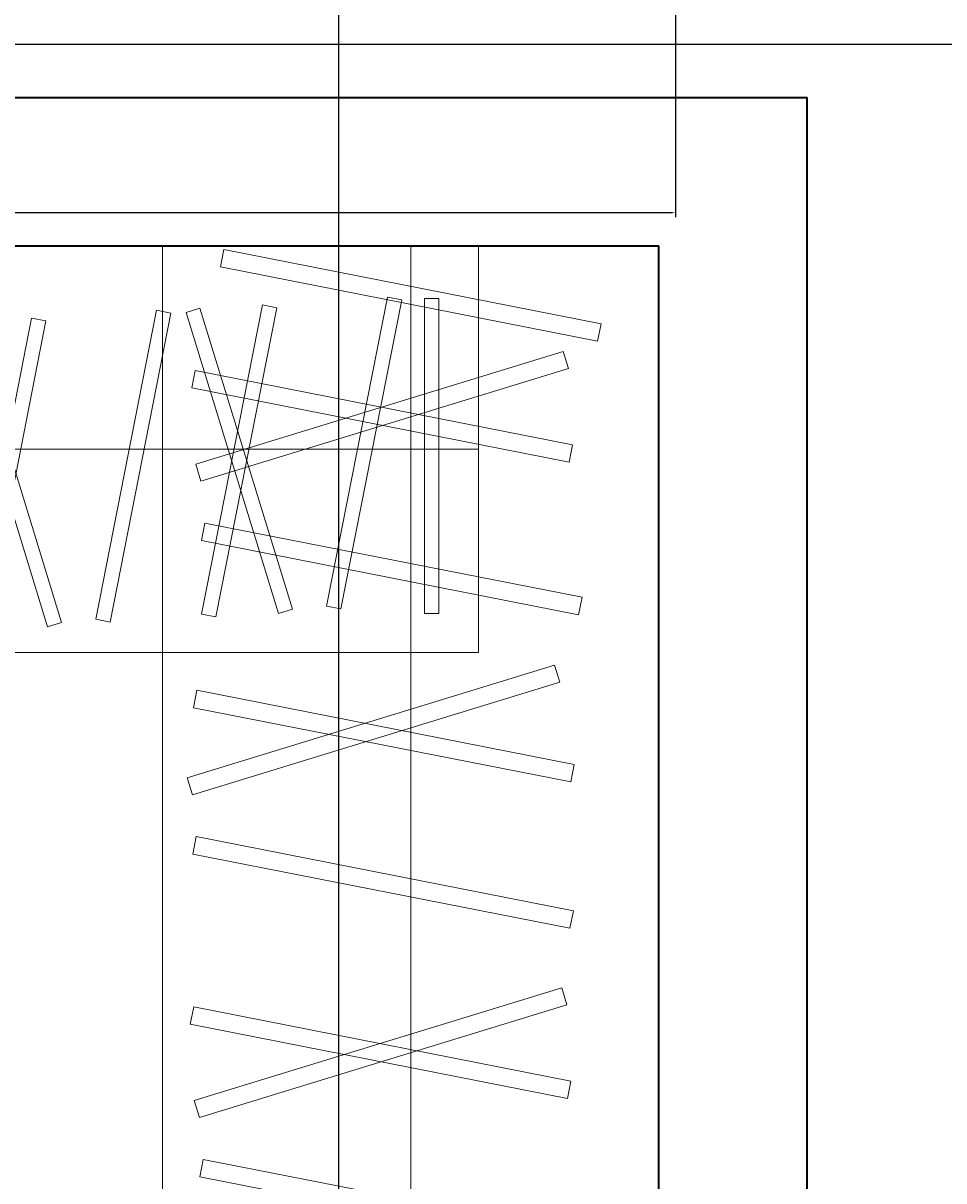
# Model space of a CAD drawing. Units: inches. Extents: x -61 to 1599, y -1316 to 257.
# Tile 66 of 204: x 203 to 240, y -213 to -166. Entities that reach past the tile are written whole.
import ezdxf

# ---------------------------------------------------------------- set-up
doc = ezdxf.new("R2010")
doc.units = ezdxf.units.IN
doc.header["$MEASUREMENT"] = 0
for name, color, linetype, lineweight in [('A-ANNO-DIMS', 2, 'Continuous', 18), ('A-FLOR-CASE', 8, 'Continuous', 18), ('WALLS', 4, 'Continuous', 35)]:
    doc.layers.add(name, color=color, linetype=linetype, lineweight=lineweight)
doc.styles.get("Standard").update_dxf_attribs({"font": 'arial.ttf'})
doc.dimstyles.get("Standard").update_dxf_attribs({"dimtxt": 0.18, "dimasz": 0.18, "dimexe": 0.18, "dimexo": 0.0625, "dimgap": 0.09, "dimtad": 0, "dimtih": 1, "dimtoh": 1, "dimdec": 0, "dimzin": 0, "dimdsep": 46, "dimlunit": 3, "dimtxsty": 'Standard', "dimcen": 0.09, "dimadec": 0, "dimazin": 0, "dimtfac": 1, "dimtdec": 0, "dimtofl": 0, "dimtmove": 0, "dimatfit": 3, "dimfxl": 1, "dimtolj": 1, "dimtzin": 0, "dimarcsym": 0})

# ---------------------------------------------------------------- blocks, each defined once
blk = doc.blocks.new('WARDROBE-HANGING')
blk.add_line((10.047, 0), (10.047, 68))
for points in [[(20.094, 0), (0, 0), (0, 68), (20.094, 68)], [(2.482, 67.852), (17.751, 64.849), (17.612, 64.142), (2.343, 67.146)], [(1.346, 59.162), (16.221, 63.731), (16.432, 63.043), (1.557, 58.474)], [(1.325, 62.957), (16.593, 59.954), (16.454, 59.247), (1.186, 62.251)], [(1.713, 56.784), (16.981, 53.781), (16.842, 53.074), (1.574, 56.078)], [(0.997, 46.467), (15.872, 51.036), (16.084, 50.348), (1.209, 45.779)], [(1.394, 50.014), (16.662, 47.011), (16.523, 46.305), (1.255, 49.308)], [(1.365, 44.09), (16.633, 41.086), (16.494, 40.38), (1.226, 43.383)], [(1.283, 33.408), (16.158, 37.977), (16.37, 37.289), (1.495, 32.72)], [(1.262, 37.203), (16.53, 34.2), (16.391, 33.493), (1.123, 36.497)], [(1.651, 31.03), (16.919, 28.027), (16.78, 27.32), (1.512, 30.324)]]:
    blk.add_lwpolyline(points, close=True)
blk = doc.blocks.new('WARDROBE-HANGING-2')
blk.add_line((55.703, 8.23), (0, 8.23))
for points in [[(55.703, 16.46), (55.703, 0), (0, 0), (0, 16.46)], [(0.121, 2.033), (2.581, 14.541), (3.16, 14.427), (0.7, 1.92)], [(44.491, 1.561), (46.952, 14.069), (47.53, 13.955), (45.07, 1.448)], [(49.548, 1.88), (52.008, 14.387), (52.587, 14.273), (50.127, 1.766)], [(54.096, 14.328), (54.096, 1.581), (53.506, 1.581), (53.506, 14.328)], [(4.131, 1.085), (6.591, 13.592), (7.17, 13.478), (4.709, 0.971)], [(9.187, 1.403), (11.648, 13.911), (12.226, 13.797), (9.766, 1.289)], [(14.733, 1.142), (17.193, 13.649), (17.772, 13.535), (15.312, 1.028)], [(19.586, 1.118), (22.047, 13.625), (22.625, 13.511), (20.165, 1.004)], [(30.284, 1.352), (32.745, 13.859), (33.323, 13.745), (30.863, 1.238)], [(40.204, 1.348), (42.664, 13.855), (43.243, 13.742), (40.782, 1.234)], [(47.6, 1.579), (43.858, 13.764), (44.421, 13.937), (48.164, 1.752)], [(7.24, 1.102), (3.497, 13.288), (4.061, 13.461), (7.804, 1.276)], [(17.639, 0.817), (13.896, 13.002), (14.46, 13.175), (18.203, 0.99)], [(28.337, 1.051), (24.594, 13.236), (25.158, 13.409), (28.901, 1.224)], [(25.228, 1.034), (27.688, 13.541), (28.267, 13.427), (25.806, 0.92)], [(38.256, 1.047), (34.513, 13.232), (35.077, 13.406), (38.82, 1.221)], [(35.147, 1.03), (37.607, 13.537), (38.186, 13.423), (35.726, 0.916)]]:
    blk.add_lwpolyline(points, close=True)
blk = doc.blocks.new('*D670')
at = {"layer": 'A-ANNO-DIMS', "color": 0, "lineweight": -2, "transparency": 16777216}
for p, q in [((145.375, -161.442), (145.375, -174.159)), ((229.375, -161.442), (229.375, -174.159)), ((145.555, -173.979), (186.47, -173.979)), ((229.195, -173.979), (188.279, -173.979))]:
    blk.add_line(p, q, dxfattribs=at)
at = {"layer": 'A-ANNO-DIMS', "color": 0, "transparency": 16777216}
for points in [[(145.555, -173.949), (145.555, -174.009), (145.375, -173.979)], [(229.195, -173.949), (229.195, -174.009), (229.375, -173.979)]]:
    blk.add_solid(points, dxfattribs=at)
at = {"layer": 'DEFPOINTS', "color": 0, "transparency": 16777216}
for p in [(145.375, -161.379), (229.375, -161.379), (229.375, -173.979)]:
    blk.add_point(p, dxfattribs=at)
at = {"layer": 'A-ANNO-DIMS', "color": 0, "transparency": 16777216, "insert": (187.375, -173.979), "char_height": 0.18, "attachment_point": 5}
blk.add_mtext('\\A1;SOFA 84 TYP.', dxfattribs=at)
blk = doc.blocks.new('*D687')
at = {"layer": 'A-ANNO-DIMS', "color": 0, "lineweight": -2, "transparency": 16777216}
for p, q in [((289.418, 181.677), (-61.077, 181.677)), ((-60.897, 181.497), (-60.897, -528.952)), ((-60.897, -1239.765), (-60.897, -529.316)), ((319.64, -1239.945), (-61.077, -1239.945))]:
    blk.add_line(p, q, dxfattribs=at)
at = {"layer": 'A-ANNO-DIMS', "color": 0, "transparency": 16777216}
for points in [[(-60.927, 181.497), (-60.867, 181.497), (-60.897, 181.677)], [(-60.927, -1239.765), (-60.867, -1239.765), (-60.897, -1239.945)]]:
    blk.add_solid(points, dxfattribs=at)
at = {"layer": 'DEFPOINTS', "color": 0, "transparency": 16777216}
for p in [(289.481, 181.677), (-60.897, -1239.945), (319.703, -1239.945)]:
    blk.add_point(p, dxfattribs=at)
at = {"layer": 'A-ANNO-DIMS', "color": 0, "transparency": 16777216, "insert": (-60.897, -529.134), "char_height": 0.18, "attachment_point": 5}
blk.add_mtext('\\A1;1421.6', dxfattribs=at)
blk = doc.blocks.new('*D699')
at = {"layer": 'A-ANNO-DIMS', "color": 0, "lineweight": -2, "transparency": 16777216}
for p, q in [((835.64, -167.169), (-61.077, -167.169)), ((-60.897, -167.349), (-60.897, -306.726)), ((-60.897, -446.466), (-60.897, -307.09)), ((841.64, -446.646), (-61.077, -446.646))]:
    blk.add_line(p, q, dxfattribs=at)
at = {"layer": 'A-ANNO-DIMS', "color": 0, "transparency": 16777216}
for points in [[(-60.927, -167.349), (-60.867, -167.349), (-60.897, -167.169)], [(-60.927, -446.466), (-60.867, -446.466), (-60.897, -446.646)]]:
    blk.add_solid(points, dxfattribs=at)
at = {"layer": 'DEFPOINTS', "color": 0, "transparency": 16777216}
for p in [(835.703, -167.169), (-60.897, -446.646), (841.703, -446.646)]:
    blk.add_point(p, dxfattribs=at)
at = {"layer": 'A-ANNO-DIMS', "color": 0, "transparency": 16777216, "insert": (-60.897, -306.908), "char_height": 0.18, "attachment_point": 5}
blk.add_mtext('\\A1;279.5', dxfattribs=at)
blk = doc.blocks.new('*D701')
at = {"layer": 'A-ANNO-DIMS', "color": 0, "lineweight": -2, "transparency": 16777216}
for p, q in [((215.752, -616.882), (215.752, 257.457)), ((215.932, 257.277), (233.924, 257.277)), ((252.702, 257.277), (234.711, 257.277)), ((252.882, -616.882), (252.882, 257.457))]:
    blk.add_line(p, q, dxfattribs=at)
at = {"layer": 'A-ANNO-DIMS', "color": 0, "transparency": 16777216}
for points in [[(215.932, 257.307), (215.932, 257.247), (215.752, 257.277)], [(252.702, 257.307), (252.702, 257.247), (252.882, 257.277)]]:
    blk.add_solid(points, dxfattribs=at)
at = {"layer": 'DEFPOINTS', "color": 0, "transparency": 16777216}
for p in [(252.882, 257.277), (215.752, -616.945), (252.882, -616.945)]:
    blk.add_point(p, dxfattribs=at)
at = {"layer": 'A-ANNO-DIMS', "color": 0, "transparency": 16777216, "insert": (234.317, 257.277), "char_height": 0.18, "attachment_point": 5}
blk.add_mtext('\\A1;37.13', dxfattribs=at)

msp = doc.modelspace()

# ---------------------------------------------------------------- linework, layer by layer
at = {"layer": 'WALLS'}
for p, q in [((119.7028, -169.3229), (234.7028, -169.3229)), ((234.7028, -282.3229), (234.7028, -169.3229)), ((165.7028, -175.3229), (228.7028, -175.3229)), ((228.7028, -282.3229), (228.7028, -175.3229))]:
    msp.add_line(p, q, dxfattribs=at)

# ---------------------------------------------------------------- block references
at = {"layer": 'A-FLOR-CASE'}
for name, p in [('WARDROBE-HANGING-2', (165.703, -191.783)), ('WARDROBE-HANGING', (208.609, -243.323))]:
    msp.add_blockref(name, p, dxfattribs=at)

# ---------------------------------------------------------------- dimensions: what is measured, and where the dimension line sits
at = {"layer": 'A-ANNO-DIMS'}
dim = msp.add_linear_dim(base=(252.8825, 257.2771), p1=(215.7521, -616.9446), p2=(252.8825, -616.9446), dimstyle='Standard', override={"dimdec": 2, "dimlfac": 1, "dimrnd": 0, "dimzin": 0, "dimdsep": 46, "dimlunit": 2}, dxfattribs=at)
dim.commit()
dim.dimension.update_dxf_attribs({"geometry": '*D701', "text_midpoint": (234.3173, 257.2771)})
for base, p1, p2, picture, middle in [((-60.8972, -1239.9446), (289.4807, 181.6771), (319.7028, -1239.9446), '*D687', (-60.8972, -529.1337)), ((-60.8972, -446.6462), (835.7028, -167.169), (841.7028, -446.6462), '*D699', (-60.8972, -306.9076))]:
    dim = msp.add_linear_dim(base=base, p1=p1, p2=p2, angle=90, dimstyle='Standard', override={"dimdec": 1, "dimlfac": 1, "dimrnd": 0, "dimzin": 0, "dimdsep": 46, "dimlunit": 2}, dxfattribs=at)
    dim.commit()
    dim.dimension.update_dxf_attribs({"geometry": picture, "text_midpoint": middle})
dim = msp.add_linear_dim(base=(229.3746, -173.9792), p1=(145.3746, -161.3792), p2=(229.3746, -161.3792), text='SOFA <> TYP.', dimstyle='Standard', override={"dimdec": 0, "dimlfac": 1, "dimrnd": 0, "dimzin": 0, "dimdsep": 46, "dimlunit": 2}, dxfattribs=at)
dim.commit()
dim.dimension.update_dxf_attribs({"geometry": '*D670', "text_midpoint": (187.3746, -173.9792)})

doc.saveas('drawing.dxf')
